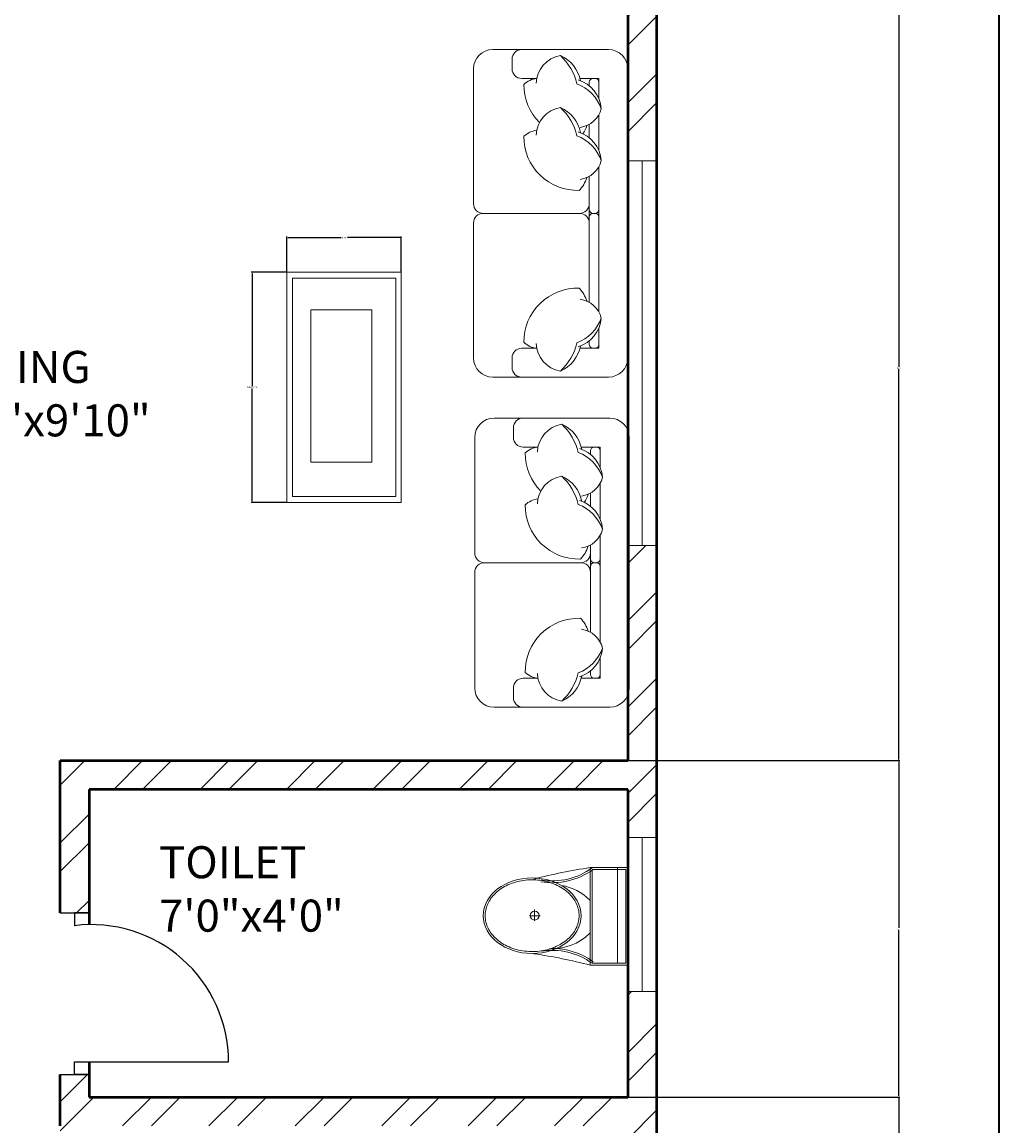
# Model space of a CAD drawing. Units: inches. Extents: x 2129 to 2642, y 1542 to 2414.
# Tile 8 of 9: x 2490 to 2642, y 2007 to 2179. Entities that reach past the tile are written whole.
import ezdxf

# ---------------------------------------------------------------- set-up
doc = ezdxf.new("R2010")
doc.units = ezdxf.units.IN
for name, color, linetype, lineweight in [('A-ANNO-DIMS', 2, 'Continuous', 18), ('A-ANNO-TTLB', 7, 'Continuous', 35), ('A-AREA-IDEN', 7, 'Continuous', 18), ('A-DOOR', 3, 'Continuous', 25), ('A-FLOR-FIXT', 9, 'Continuous', 18), ('A-FURN', 8, 'Continuous', 18), ('A-GLAZ', 4, 'Continuous', 18), ('A-WALL', 7, 'Continuous', 50), ('A-WALL-PATT', 252, 'Continuous', 13)]:
    doc.layers.add(name, color=color, linetype=linetype, lineweight=lineweight)
doc.styles.get("Standard").update_dxf_attribs({"font": 'arial.ttf'})
doc.dimstyles.get("Standard").update_dxf_attribs({"dimtxt": 0.18, "dimasz": 0.18, "dimexe": 0.18, "dimexo": 0.0625, "dimgap": 0.09, "dimtad": 0, "dimtih": 1, "dimtoh": 1, "dimdec": 4, "dimzin": 0, "dimdsep": 46, "dimtxsty": 'Standard', "dimcen": 0.09, "dimadec": 0, "dimazin": 0, "dimtfac": 1, "dimtdec": 4, "dimtofl": 0, "dimtmove": 0, "dimatfit": 3, "dimfxl": 1, "dimtolj": 1, "dimtzin": 0, "dimarcsym": 0})

# ---------------------------------------------------------------- blocks, each defined once
blk = doc.blocks.new('A$C31115884')
for p, q in [((283.1, 497.7), (223.4, 497.7)), ((257.5, 466.4), (257.5, 523.2)), ((0, 200), (0, 0)), ((520, 200), (0, 200)), ((10, 190), (10, 10)), ((510, 190), (10, 190)), ((510, 10), (510, 190)), ((520, 0), (520, 200)), ((510, 54.5), (0, 54.5)), ((10, 10), (510, 10)), ((0, 0), (520, 0))]:
    blk.add_line(p, q)
blk.add_circle((255.6, 496.4), 23.6)
for centre, radius, start, end in [((2777.7, -204.6), 2807, 165.4549, 171.71327), ((3237, 905), 2807, 188.28673, 194.5451), ((-294.5, 403.3), 364.7, 324.20913, 9.34987), ((-294.5, 403.3), 374.7, 324.20913, 9.34987), ((139.5, 406.2), 293.5, 315.84364, 2.65635), ((805.8, 403.3), 364.7, 170.65013, 215.79087), ((383.6, 406.2), 293.5, 190.27735, 224.15636), ((805.8, 403.3), 374.7, 179.20365, 215.79087)]:
    blk.add_arc(centre, radius, start, end)
blk.add_ellipse((256.2, 509.9), major_axis=(0, -260.7), ratio=0.772727)
blk.add_open_spline([(256.2, 259.2), (263.1, 259.2), (270, 259.7), (287.8, 262.3), (298.7, 265.1), (319.9, 273.1), (330.2, 278.4), (350.1, 291.1), (359.7, 298.7), (377.7, 315.9), (386.2, 325.5), (401.7, 346.6), (408.8, 358.1), (421.3, 382.5), (426.8, 395.5), (435.9, 422.4), (439.5, 436.4), (444.8, 465.1), (446.5, 479.7), (447.9, 509.2), (447.6, 524), (445, 553.3), (442.7, 567.8), (436.3, 596), (432.1, 609.7), (421.9, 636), (416, 648.6), (402.5, 672.1), (395, 683), (378.6, 703), (369.8, 712.1), (351.1, 728), (341.3, 734.8), (320.9, 746.2), (310.4, 750.7), (288.9, 757.3), (278, 759.4), (256, 761), (245, 760.6), (223.1, 757.2), (212.3, 754.3), (191.1, 746.1), (180.8, 740.7), (160.9, 727.8), (151.4, 720.1), (133.5, 702.7), (125.1, 693), (109.6, 671.7), (102.6, 660.2), (90.2, 635.7), (84.9, 622.7), (76, 595.6), (72.4, 581.6), (67.2, 552.9), (65.6, 538.2), (64.4, 508.8), (64.8, 494), (67.5, 464.7), (69.9, 450.2), (76.6, 422), (80.8, 408.3), (91.1, 382.2), (97.2, 369.7), (110.8, 346.3), (118.4, 335.4), (134.8, 315.6), (143.7, 306.7), (162.4, 290.9), (172.3, 284.2), (192.8, 273), (203.3, 268.6), (224.8, 262.2), (235.8, 260.2), (249.9, 259.3), (253, 259.2), (256.2, 259.2)], degree=3, knots=[0, 0, 0, 0, 0.110105, 0.110105, 0.285049, 0.285049, 0.459994, 0.459994, 0.634938, 0.634938, 0.809882, 0.809882, 0.984827, 0.984827, 1.159771, 1.159771, 1.334715, 1.334715, 1.50966, 1.50966, 1.684604, 1.684604, 1.859549, 1.859549, 2.034493, 2.034493, 2.209437, 2.209437, 2.384382, 2.384382, 2.559326, 2.559326, 2.73427, 2.73427, 2.909215, 2.909215, 3.084159, 3.084159, 3.259103, 3.259103, 3.434048, 3.434048, 3.608992, 3.608992, 3.783936, 3.783936, 3.958881, 3.958881, 4.133825, 4.133825, 4.30877, 4.30877, 4.483714, 4.483714, 4.658658, 4.658658, 4.833603, 4.833603, 5.008547, 5.008547, 5.183491, 5.183491, 5.358436, 5.358436, 5.53338, 5.53338, 5.708324, 5.708324, 5.883269, 5.883269, 6.058213, 6.058213, 6.233158, 6.233158, 6.283185, 6.283185, 6.283185, 6.283185])
blk = doc.blocks.new('TABLE-COFFEE')
for points in [[(0, 35.92), (17.84, 35.92), (17.84, 0), (0, 0)], [(0.86, 34.99), (17.01, 34.99), (17.01, 0.93), (0.86, 0.93)], [(3.74, 30.05), (13.25, 30.05), (13.25, 6.3), (3.74, 6.3)]]:
    blk.add_lwpolyline(points, close=True)
blk = doc.blocks.new('WIN-60-B')
for p, q in [((4.5, 60), (0, 60)), ((0, 60), (2.25, 60)), ((2.25, 60), (2.25, 0)), ((2.25, 0), (0, 0)), ((0, 0), (4.5, 0))]:
    blk.add_line(p, q)
blk = doc.blocks.new('*D32')
at = {"layer": 'A-ANNO-DIMS', "color": 0, "lineweight": -2, "transparency": 16777216}
for p, q in [((2531.18, 2140.41), (2525.67, 2140.41)), ((2525.85, 2140.23), (2525.85, 2122.64)), ((2525.85, 2104.67), (2525.85, 2122.27)), ((2531.18, 2104.49), (2525.67, 2104.49))]:
    blk.add_line(p, q, dxfattribs=at)
at = {"layer": 'A-ANNO-DIMS', "color": 0, "transparency": 16777216}
for points in [[(2525.82, 2140.23), (2525.88, 2140.23), (2525.85, 2140.41)], [(2525.82, 2104.67), (2525.88, 2104.67), (2525.85, 2104.49)]]:
    blk.add_solid(points, dxfattribs=at)
at = {"layer": 'Defpoints', "color": 0, "transparency": 16777216}
for p in [(2525.85, 2140.41), (2531.24, 2140.41), (2531.24, 2104.49)]:
    blk.add_point(p, dxfattribs=at)
at = {"layer": 'A-ANNO-DIMS', "color": 0, "transparency": 16777216, "insert": (2525.85, 2122.45), "char_height": 0.18, "attachment_point": 5}
blk.add_mtext('\\A1;TABLE 36 TYP.', dxfattribs=at)
blk = doc.blocks.new('*D33')
at = {"layer": 'A-ANNO-DIMS', "color": 0, "lineweight": -2, "transparency": 16777216}
for p, q in [((2531.24, 2140.48), (2531.24, 2145.98)), ((2531.42, 2145.8), (2539.64, 2145.8)), ((2548.91, 2145.8), (2540.68, 2145.8)), ((2549.09, 2140.48), (2549.09, 2145.98))]:
    blk.add_line(p, q, dxfattribs=at)
at = {"layer": 'A-ANNO-DIMS', "color": 0, "transparency": 16777216}
for points in [[(2531.42, 2145.83), (2531.42, 2145.77), (2531.24, 2145.8)], [(2548.91, 2145.83), (2548.91, 2145.77), (2549.09, 2145.8)]]:
    blk.add_solid(points, dxfattribs=at)
at = {"layer": 'Defpoints', "color": 0, "transparency": 16777216}
for p in [(2549.09, 2145.8), (2531.24, 2140.41), (2549.09, 2140.41)]:
    blk.add_point(p, dxfattribs=at)
at = {"layer": 'A-ANNO-DIMS', "color": 0, "transparency": 16777216, "insert": (2540.16, 2145.8), "char_height": 0.18, "attachment_point": 5}
blk.add_mtext('\\A1;18 TYP.', dxfattribs=at)
blk = doc.blocks.new('*D42')
at = {"layer": 'A-ANNO-DIMS', "color": 0, "lineweight": -2, "transparency": 16777216}
for p, q in [((2584.47, 2011.72), (2626.83, 2011.72)), ((2626.65, 2011.54), (2626.65, 1976.65)), ((2626.65, 1941.4), (2626.65, 1976.29)), ((2584.47, 1941.22), (2626.83, 1941.22))]:
    blk.add_line(p, q, dxfattribs=at)
at = {"layer": 'A-ANNO-DIMS', "color": 0, "transparency": 16777216}
for points in [[(2626.62, 2011.54), (2626.68, 2011.54), (2626.65, 2011.72)], [(2626.62, 1941.4), (2626.68, 1941.4), (2626.65, 1941.22)]]:
    blk.add_solid(points, dxfattribs=at)
at = {"layer": 'Defpoints', "color": 0, "transparency": 16777216}
for p in [(2584.4, 2011.72), (2626.65, 2011.72), (2584.4, 1941.22)]:
    blk.add_point(p, dxfattribs=at)
at = {"layer": 'A-ANNO-DIMS', "color": 0, "transparency": 16777216, "insert": (2626.65, 1976.47), "char_height": 0.18, "attachment_point": 5}
blk.add_mtext('\\A1;70.5', dxfattribs=at)
blk = doc.blocks.new('*D43')
at = {"layer": 'A-ANNO-DIMS', "color": 0, "lineweight": -2, "transparency": 16777216}
for p, q in [((2584.47, 2064.22), (2626.83, 2064.22)), ((2626.65, 2064.04), (2626.65, 2038.15)), ((2626.65, 2011.9), (2626.65, 2037.79)), ((2584.47, 2011.72), (2626.83, 2011.72))]:
    blk.add_line(p, q, dxfattribs=at)
at = {"layer": 'A-ANNO-DIMS', "color": 0, "transparency": 16777216}
for points in [[(2626.62, 2064.04), (2626.68, 2064.04), (2626.65, 2064.22)], [(2626.62, 2011.9), (2626.68, 2011.9), (2626.65, 2011.72)]]:
    blk.add_solid(points, dxfattribs=at)
at = {"layer": 'Defpoints', "color": 0, "transparency": 16777216}
for p in [(2584.4, 2064.22), (2626.65, 2064.22), (2584.4, 2011.72)]:
    blk.add_point(p, dxfattribs=at)
at = {"layer": 'A-ANNO-DIMS', "color": 0, "transparency": 16777216, "insert": (2626.65, 2037.97), "char_height": 0.18, "attachment_point": 5}
blk.add_mtext('\\A1;52.5', dxfattribs=at)
blk = doc.blocks.new('*D44')
at = {"layer": 'A-ANNO-DIMS', "color": 0, "lineweight": -2, "transparency": 16777216}
for p, q in [((2584.47, 2186.72), (2626.83, 2186.72)), ((2626.65, 2186.54), (2626.65, 2125.65)), ((2626.65, 2064.4), (2626.65, 2125.29)), ((2584.47, 2064.22), (2626.83, 2064.22))]:
    blk.add_line(p, q, dxfattribs=at)
at = {"layer": 'A-ANNO-DIMS', "color": 0, "transparency": 16777216}
for points in [[(2626.62, 2186.54), (2626.68, 2186.54), (2626.65, 2186.72)], [(2626.62, 2064.4), (2626.68, 2064.4), (2626.65, 2064.22)]]:
    blk.add_solid(points, dxfattribs=at)
at = {"layer": 'Defpoints', "color": 0, "transparency": 16777216}
for p in [(2584.4, 2186.72), (2626.65, 2186.72), (2584.4, 2064.22)]:
    blk.add_point(p, dxfattribs=at)
at = {"layer": 'A-ANNO-DIMS', "color": 0, "transparency": 16777216, "insert": (2626.65, 2125.47), "char_height": 0.18, "attachment_point": 5}
blk.add_mtext('\\A1;122.5', dxfattribs=at)

msp = doc.modelspace()

# ---------------------------------------------------------------- hatches: boundary and pattern name
at = {"layer": 'A-WALL-PATT'}
h = msp.add_hatch(dxfattribs=at)
h.set_pattern_fill('ANSI32', color=256)
h.paths.add_polyline_path([(2306.2606, 2305.9717), (2306.2606, 2308.2217), (2276.3515, 2308.2217), (2276.3515, 2303.7217), (2306.2606, 2303.7217)])
h.paths.add_polyline_path([(2216.3515, 2305.9717), (2216.3515, 2308.2217), (2186.9043, 2308.2217), (2186.9043, 2278.1696), (2191.4043, 2278.1696), (2191.4043, 2303.7217), (2216.3515, 2303.7217)])
h.paths.add_polyline_path([(2339.9043, 2335.7217), (2362.1938, 2335.7217), (2362.1938, 2340.2217), (2335.4043, 2340.2217), (2335.4043, 2308.2217), (2329.3487, 2308.2217), (2329.3487, 2305.9717), (2329.3487, 2303.7217), (2335.4043, 2303.7217), (2335.4043, 2186.7217), (2329.4345, 2186.7217), (2329.4345, 2182.2217), (2335.4043, 2182.2217), (2335.4043, 2174.7178), (2339.9043, 2174.7178), (2339.9043, 2182.2217), (2339.9043, 2303.7217)])
h.paths.add_polyline_path([(2440.4043, 2340.2217), (2411.654, 2340.2217), (2411.654, 2335.7217), (2435.9043, 2335.7217), (2435.9043, 2303.7217), (2435.9043, 2182.2217), (2435.9043, 2174.1935), (2438.1543, 2174.1935), (2440.4043, 2174.1935), (2440.4043, 2182.2217), (2444.653, 2182.2217), (2444.653, 2184.4717), (2444.653, 2186.7217), (2440.4043, 2186.7217), (2440.4043, 2303.7217), (2445.8547, 2303.7217), (2445.8547, 2308.2217), (2440.4043, 2308.2217)])
h.paths.add_polyline_path([(2498.2381, 2308.2217), (2470.3901, 2308.2217), (2470.3901, 2303.7217), (2498.2381, 2303.7217), (2498.2381, 2305.9717)])
h.paths.add_polyline_path([(2588.9043, 2308.2217), (2586.9043, 2308.2217), (2558.2381, 2308.2217), (2558.2381, 2303.7217), (2584.4043, 2303.7217), (2584.4043, 2279.1087), (2588.9043, 2279.1087)])
h.paths.add_polyline_path([(2588.9043, 2219.1087), (2584.4043, 2219.1087), (2584.4043, 2186.7217), (2478.0667, 2186.7217), (2478.0667, 2182.2217), (2584.4043, 2182.2217), (2584.4043, 2157.7883), (2588.9043, 2157.7883)])
h.paths.add_polyline_path([(2588.9043, 2097.7883), (2584.6063, 2097.7883), (2584.6063, 2075.5462, -0.09241561), (2584.4043, 2074.4627), (2584.4043, 2064.2217), (2495.9043, 2064.2217), (2495.9043, 2040.4611), (2500.4043, 2040.4611), (2500.4043, 2059.7217), (2584.4043, 2059.7217), (2584.4043, 2052.2164), (2588.9043, 2052.2164)])
h.paths.add_polyline_path([(2588.9043, 2028.2164), (2584.4043, 2028.2164), (2584.4043, 2011.7217), (2500.4043, 2011.7217), (2500.4043, 2015.243), (2498.1543, 2015.243), (2495.9043, 2015.243), (2495.9043, 2007.2217), (2495.9043, 2003.7597), (2500.4043, 2003.7597), (2500.4043, 2007.2217), (2584.4043, 2007.2217), (2584.4043, 1992.1997), (2588.9043, 1992.1997)])
h.paths.add_polyline_path([(2588.9043, 1956.1997), (2584.4043, 1956.1997), (2584.4043, 1941.2217), (2500.4043, 1941.2217), (2500.4043, 1985.1493), (2498.1543, 1985.1493), (2495.9043, 1985.1493), (2495.9043, 1941.2217), (2435.9043, 1941.2217), (2435.9043, 1930.3963), (2440.4043, 1930.3963), (2440.4043, 1936.7217), (2584.4043, 1936.7217), (2584.4043, 1909.8406), (2588.9043, 1909.8406)])
h.paths.add_polyline_path([(2588.9043, 1849.8406), (2584.4043, 1849.8406), (2584.4043, 1801.3526), (2588.9043, 1801.3526)])
h.paths.add_polyline_path([(2584.4043, 1828.7217), (2495.9043, 1828.7217), (2440.4043, 1828.7217), (2440.4043, 1905.2159), (2438.1543, 1905.2159), (2435.9043, 1905.2159), (2435.9043, 1828.7217), (2428.9101, 1828.7217), (2428.9101, 1824.2217), (2584.4043, 1824.2217)])
h.paths.add_polyline_path([(2588.9043, 1741.3526), (2584.4043, 1741.3526), (2584.4043, 1704.2217), (2468.3173, 1704.2217), (2468.3173, 1701.9717), (2468.3173, 1699.7217), (2588.9043, 1699.7217)])
h.paths.add_polyline_path([(2442.4043, 1761.7217), (2435.0216, 1761.7217), (2435.0216, 1757.2217), (2437.9043, 1757.2217), (2437.9043, 1665.7217), (2442.4043, 1665.7217), (2442.4043, 1667.7217), (2442.4043, 1699.7217), (2446.6907, 1699.7217), (2446.6907, 1701.9717), (2446.6907, 1704.2217), (2442.4043, 1704.2217)])
h.paths.add_polyline_path([(2390.4043, 1757.2217), (2410.8996, 1757.2217), (2410.8996, 1761.7217), (2360.1741, 1761.7217), (2360.1741, 1759.4717), (2360.1741, 1757.2217), (2385.9043, 1757.2217), (2385.9043, 1674.8326), (2390.4043, 1674.8326)])
h.paths.add_polyline_path([(2337.9043, 1757.2217), (2340.3592, 1757.2217), (2340.3592, 1759.4717), (2340.3592, 1761.7217), (2333.4043, 1761.7217), (2333.4043, 1704.2217), (2327.381, 1704.2217), (2327.381, 1701.9717), (2327.381, 1699.7217), (2333.4043, 1699.7217), (2333.4043, 1665.7217), (2337.9043, 1665.7217)])
h.paths.add_polyline_path([(2191.4043, 1743.4804), (2186.9043, 1743.4804), (2186.9043, 1699.7217), (2188.9043, 1699.7217), (2191.4043, 1699.7217), (2306.5617, 1699.7217), (2306.5617, 1704.2217), (2191.4043, 1704.2217)])
h.paths.add_polyline_path([(2191.4043, 1859.8992), (2186.9043, 1859.8992), (2186.9043, 1803.4804), (2189.1543, 1803.4804), (2191.4043, 1803.4804)])
h.paths.add_polyline_path([(2352.5445, 1828.7217), (2191.4043, 1828.7217), (2191.4043, 1824.2217), (2333.4043, 1824.2217), (2352.5445, 1824.2217), (2352.5445, 1826.4717)])
h.paths.add_polyline_path([(2390.4043, 2085.328), (2385.9043, 2085.328), (2385.9043, 1828.7217), (2381.9668, 1828.7217), (2381.9668, 1826.4717), (2381.9668, 1824.2217), (2385.9043, 1824.2217), (2385.9043, 1761.7217), (2390.4043, 1761.7217), (2390.4043, 1824.2217), (2394.1868, 1824.2217), (2394.1868, 1827.6339), (2394.1868, 1828.7217), (2390.4043, 1828.7217)])
h.paths.add_polyline_path([(2339.9043, 1941.2217), (2335.4043, 1941.2217), (2279.9043, 1941.2217), (2279.9043, 1981.3432), (2277.6543, 1981.3432), (2275.4043, 1981.3432), (2275.4043, 1941.2217), (2191.4043, 1941.2217), (2191.4043, 1958.1079), (2186.9043, 1958.1079), (2186.9043, 1919.8992), (2189.1543, 1919.8992), (2191.4043, 1919.8992), (2191.4043, 1936.7217), (2279.9043, 1936.7217), (2335.4043, 1936.7217), (2335.4043, 1931.1382), (2339.9043, 1931.1382)])
h.paths.add_polyline_path([(2339.9043, 1902.7544), (2337.6543, 1902.7544), (2335.4043, 1902.7544), (2335.4043, 1828.7217), (2339.9043, 1828.7217)])
h.paths.add_polyline_path([(2279.9043, 2015.263), (2277.6543, 2015.263), (2275.4043, 2015.263), (2275.4043, 2011.7217), (2191.4043, 2011.7217), (2191.4043, 2026.6781), (2186.9043, 2026.6781), (2186.9043, 1994.1079), (2189.1543, 1994.1079), (2191.4043, 1994.1079), (2191.4043, 2007.2217), (2275.4043, 2007.2217), (2275.4043, 2003.2288), (2279.9043, 2003.2288), (2279.9043, 2007.2217)])
h.paths.add_polyline_path([(2296.0216, 2186.7217), (2191.4043, 2186.7217), (2191.4043, 2218.1696), (2186.9043, 2218.1696), (2186.9043, 2158.4509), (2191.4043, 2158.4509), (2191.4043, 2182.2217), (2296.0216, 2182.2217), (2296.0216, 2184.4717)])
h.paths.add_polyline_path([(2191.4043, 2098.4509), (2189.1543, 2098.4509), (2186.9043, 2098.4509), (2186.9043, 2050.6781), (2189.0487, 2050.6781), (2191.4043, 2050.6781), (2191.4043, 2059.7217), (2275.4043, 2059.7217), (2275.4043, 2038.4133), (2279.9043, 2038.4133), (2279.9043, 2064.2217), (2191.4043, 2064.2217)])
h.paths.add_polyline_path([(2268.3923, 1605.9386), (2516.3159, 1605.9386), (2516.3159, 1643.0314), (2268.3923, 1643.0314)], flags=9)
h.paths.add_polyline_path([(2399.6079, 1710.4489), (2428.8405, 1710.4489), (2428.8405, 1729.1062), (2399.6079, 1729.1062)], flags=9)
h.paths.add_polyline_path([(2342.1483, 1708.9956), (2371.3809, 1708.9956), (2371.3809, 1727.653), (2342.1483, 1727.653)], flags=9)
h.paths.add_polyline_path([(2200.7404, 1677.2519), (2282.3059, 1677.2519), (2282.3059, 1687.5555), (2200.7404, 1687.5555)], flags=9)
h.paths.add_polyline_path([(2209.8153, 1704.7448), (2250.627, 1704.7448), (2250.627, 1723.4021), (2209.8153, 1723.4021)], flags=25)
h.paths.add_polyline_path([(2213.9996, 1911.284), (2252.84, 1911.284), (2252.84, 1929.9413), (2213.9996, 1929.9413)], flags=9)
h.paths.add_polyline_path([(2210.8865, 1962.0987), (2244.0447, 1962.0987), (2244.0447, 1980.7561), (2210.8865, 1980.7561)], flags=25)
h.paths.add_polyline_path([(2219.0745, 2037.6131), (2248.2321, 2037.6131), (2248.2321, 2056.2705), (2219.0745, 2056.2705)], flags=9)
h.paths.add_polyline_path([(2379.9702, 2099.0686), (2409.3767, 2099.0686), (2409.3767, 2117.7259), (2379.9702, 2117.7259)], flags=9)
h.paths.add_polyline_path([(2375.9312, 2160.3752), (2405.3173, 2160.3752), (2405.3173, 2179.0325), (2375.9312, 2179.0325)], flags=9)
h.paths.add_polyline_path([(2269.5058, 2112.1824), (2310.3175, 2112.1824), (2310.3175, 2130.8397), (2269.5058, 2130.8397)], flags=9)
h.paths.add_polyline_path([(2209.6567, 2193.667), (2248.4971, 2193.667), (2248.4971, 2212.3243), (2209.6567, 2212.3243)], flags=25)
h.paths.add_polyline_path([(2491.6289, 1675.447), (2573.1944, 1675.447), (2573.1944, 1685.7506), (2491.6289, 1685.7506)], flags=9)
h.paths.add_polyline_path([(2492.0585, 1710.4489), (2530.8989, 1710.4489), (2530.8989, 1729.1062), (2492.0585, 1729.1062)], flags=25)
h.paths.add_polyline_path([(2495.6634, 1908.8646), (2534.5038, 1908.8646), (2534.5038, 1927.522), (2495.6634, 1927.522)], flags=9)
h.paths.add_polyline_path([(2516.7779, 1955.9942), (2549.9362, 1955.9942), (2549.9362, 1974.6516), (2516.7779, 1974.6516)], flags=25)
h.paths.add_polyline_path([(2509.7444, 2034.6896), (2538.902, 2034.6896), (2538.902, 2053.347), (2509.7444, 2053.347)], flags=9)
h.paths.add_polyline_path([(2467.8454, 2111.9593), (2508.6571, 2111.9593), (2508.6571, 2130.6167), (2467.8454, 2130.6167)], flags=9)
h.paths.add_polyline_path([(2528.5267, 2189.1742), (2567.3671, 2189.1742), (2567.3671, 2207.8316), (2528.5267, 2207.8316)], flags=25)
h.paths.add_polyline_path([(2483.7603, 2319.9841), (2557.5563, 2319.9841), (2557.5563, 2330.2877), (2483.7603, 2330.2877)], flags=9)
h.paths.add_polyline_path([(2204.078, 2317.0445), (2277.874, 2317.0445), (2277.874, 2327.3481), (2204.078, 2327.3481)], flags=9)

# ---------------------------------------------------------------- linework, layer by layer
at = {"layer": 'A-ANNO-TTLB'}
msp.add_lwpolyline([(2129.4387, 2413.7704), (2642.2731, 2413.7704), (2642.2731, 1542.3836), (2129.4387, 1542.3836)], close=True, dxfattribs=at)
at = {"layer": 'A-DOOR'}
for p, q in [((2495.9043, 2040.4611), (2500.4043, 2040.4611)), ((2500.4043, 2040.4611), (2498.1543, 2040.4611)), ((2498.1543, 2040.4611), (2498.1543, 2038.4611)), ((2498.1543, 2015.243), (2498.1543, 2017.243)), ((2498.1543, 2017.243), (2522.1543, 2017.243)), ((2495.9043, 2015.243), (2500.4043, 2015.243)), ((2500.4043, 2015.243), (2498.1543, 2015.243))]:
    msp.add_line(p, q, dxfattribs=at)
msp.add_arc((2500.775, 2017.243), 21.3793, 0, 97.041006, dxfattribs=at)
at = {"layer": 'A-FURN', "ltscale": 0.03}
for points in [[(2560.3497, 2148.0866, -0.41421356), (2561.8532, 2149.59, -0.41421356), (2560.3497, 2151.0935), (2560.3497, 2172.1412, -0.41421356), (2563.3566, 2175.1481), (2581.3975, 2175.1481, -0.41421356), (2584.4043, 2172.1412), (2584.4043, 2127.0388, -0.41421356), (2581.3975, 2124.032), (2563.3566, 2124.032, -0.41421356), (2560.3497, 2127.0388), (2560.3497, 2148.0866, -0.41421356), (2561.8532, 2149.59, -0.41421356), (2560.3497, 2151.0935)], [(2560.5517, 2093.5871, -0.41421356), (2562.0551, 2095.0905, -0.41421356), (2560.5517, 2096.594), (2560.5517, 2114.6349, -0.41421356), (2563.5585, 2117.6417), (2581.5995, 2117.6417, -0.41421356), (2584.6063, 2114.6349), (2584.6063, 2075.5462, -0.41421356), (2581.5995, 2072.5394), (2563.5585, 2072.5394, -0.41421356), (2560.5517, 2075.5462), (2560.5517, 2093.5871, -0.41421356), (2562.0551, 2095.0905, -0.41421356), (2560.5517, 2096.594)]]:
    msp.add_lwpolyline(points, format="xyb", dxfattribs=at)
at = {"layer": 'A-FURN'}
for points in [[(2570.1961, 2170.6378), (2567.8668, 2170.6378, -0.41421356), (2566.3634, 2172.1412), (2566.3634, 2173.6446, -0.41421356), (2567.8668, 2175.1481)], [(2570.1052, 2169.8833, -0.35677236), (2573.8947, 2174.1912, -0.24954205), (2577.0176, 2170.2879, 9.61688035)], [(2573.8947, 2174.1912, -0.14772988), (2576.4784, 2169.7972, -0.21334276), (2580.268, 2165.9201, -0.17866181)], [(2570.1968, 2170.6411, 0.16554063), (2568.2104, 2169.711, 0.20023115), (2570.6297, 2163.743, 0.12152332)], [(2576.6844, 2170.4042, -0.30666349), (2580.268, 2165.9201, -0.30632997), (2576.9952, 2162.9907, 0.87284716)], [(2579.8941, 2167.4751), (2579.8941, 2170.6378), (2576.9395, 2170.6378, -0.41421356)], [(2578.3907, 2169.4905), (2578.3907, 2170.0365, -0.41421356), (2578.9921, 2170.6378), (2579.2927, 2170.6378, -0.41421356), (2579.8941, 2170.0365)], [(2579.8941, 2170.0365), (2579.8941, 2167.4751, -0.41421356)], [(2570.1052, 2161.7845, -0.35677236), (2573.8947, 2166.0924, -0.24954205), (2577.0176, 2162.1891, 9.61688035)], [(2573.8947, 2166.0924, -0.14772988), (2576.4784, 2161.6984, -0.21334276), (2580.268, 2157.8213, -0.17866181)], [(2579.8941, 2164.9739), (2579.8941, 2159.3762, -0.41421356)], [(2577.4223, 2162.0114, 0.07186538), (2578.01, 2163.2719, -7.11546429)], [(2578.3907, 2161.3917), (2578.3907, 2163.4601, -0.41421356)], [(2570.1968, 2162.5423, 0.16554063), (2568.2104, 2161.6122, 0.42598917), (2576.8229, 2153.1687, 0.12152332), (2578.01, 2155.1731, -7.11546429)], [(2576.6844, 2162.3054, -0.30666349), (2580.268, 2157.8213, -0.30632997), (2576.9952, 2154.8919, 0.87284716)], [(2579.8941, 2156.8751), (2579.8941, 2150.1914, -0.41421356), (2579.2927, 2149.59), (2578.9921, 2149.59, -0.41421356), (2578.3907, 2150.1914), (2578.3907, 2155.3612, -0.41421356)], [(2578.3907, 2151.0935, -0.41421356), (2576.8873, 2149.59), (2561.8532, 2149.59, -0.41421356)], [(2578.3907, 2151.0935, -0.41421356), (2576.8873, 2149.59)], [(2578.3907, 2148.0866, 0.41421356), (2576.8873, 2149.59), (2561.8532, 2149.59, 0.41421356)], [(2578.3907, 2148.0866, 0.41421356), (2576.8873, 2149.59)], [(2579.8941, 2134.2062), (2579.8941, 2148.9887, 0.41421356), (2579.2927, 2149.59), (2578.9921, 2149.59, 0.41421356), (2578.3907, 2148.9887), (2578.3907, 2135.72, 0.41421356)], [(2570.1968, 2128.539, -0.16554063), (2568.2104, 2129.469, -0.42598917), (2576.8229, 2137.9125, -0.12152332), (2578.01, 2135.9082, 7.11546429)], [(2576.6844, 2128.7758, 0.30666349), (2580.268, 2133.26, 0.30632997), (2576.9952, 2136.1893, -0.87284716)], [(2573.8947, 2124.9888, 0.14772988), (2576.4784, 2129.3829, 0.21334276), (2580.268, 2133.26, 0.17866181)], [(2579.8941, 2129.1436), (2579.8941, 2131.705, 0.41421356)], [(2567.8668, 2124.032, -0.41421356), (2566.3634, 2125.5354), (2566.3634, 2127.0388, -0.41421356), (2567.8668, 2128.5423), (2570.1961, 2128.5423)], [(2570.1052, 2129.2967, 0.35677236), (2573.8947, 2124.9888, 0.24954205), (2577.0176, 2128.8922, -9.61688035)], [(2578.3907, 2129.6895), (2578.3907, 2129.1436, 0.41421356), (2578.9921, 2128.5423), (2579.2927, 2128.5423, 0.41421356), (2579.8941, 2129.1436)], [(2570.3981, 2113.1315), (2568.0688, 2113.1315, -0.41421356), (2566.5654, 2114.6349), (2566.5654, 2116.1383, -0.41421356), (2568.0688, 2117.6417)], [(2570.3071, 2112.377, -0.35677236), (2574.0967, 2116.6849, -0.24954205), (2577.2195, 2112.7816, 9.61688035)], [(2574.0967, 2116.6849, -0.14772988), (2576.6804, 2112.2909, -0.21334276), (2580.4699, 2108.4138, -0.17866181)], [(2570.3988, 2113.1348, 0.16554063), (2568.4124, 2112.2047, 0.20023115), (2570.8316, 2106.2367, 0.12152332)], [(2580.0961, 2109.9687), (2580.0961, 2113.1315), (2577.1415, 2113.1315, -0.41421356)], [(2578.5927, 2111.9842), (2578.5927, 2112.5301, -0.41421356), (2579.194, 2113.1315), (2579.4947, 2113.1315, -0.41421356), (2580.0961, 2112.5301)], [(2576.8863, 2112.8979, -0.30666349), (2580.4699, 2108.4138, -0.30632997), (2577.1972, 2105.4844, 0.87284716)], [(2580.0961, 2112.5301), (2580.0961, 2109.9687, -0.41421356)], [(2570.3071, 2104.2782, -0.35677236), (2574.0967, 2108.5861, -0.24954205), (2577.2195, 2104.6827, 9.61688035)], [(2574.0967, 2108.5861, -0.14772988), (2576.6804, 2104.192, -0.21334276), (2580.4699, 2100.3149, -0.17866181)], [(2580.0961, 2107.4676), (2580.0961, 2101.8699, -0.41421356)], [(2570.3988, 2105.0359, 0.16554063), (2568.4124, 2104.1059, 0.42598917), (2577.0249, 2095.6624, 0.12152332), (2578.212, 2097.6667, -7.11546429)], [(2576.8863, 2104.7991, -0.30666349), (2580.4699, 2100.3149, -0.30632997), (2577.1972, 2097.3856, 0.87284716)], [(2577.6243, 2104.5051, 0.07186538), (2578.212, 2105.7656, -7.11546429)], [(2578.5927, 2103.8854), (2578.5927, 2105.9538, -0.41421356)], [(2580.0961, 2099.3688), (2580.0961, 2095.6919, -0.41421356), (2579.4947, 2095.0905), (2579.194, 2095.0905, -0.41421356), (2578.5927, 2095.6919), (2578.5927, 2097.8549, -0.41421356)], [(2578.5927, 2096.594, -0.41421356), (2577.0893, 2095.0905), (2562.0551, 2095.0905, -0.41421356)], [(2578.5927, 2096.594, -0.41421356), (2577.0893, 2095.0905)], [(2578.5927, 2093.5871, 0.41421356), (2577.0893, 2095.0905), (2562.0551, 2095.0905, 0.41421356)], [(2578.5927, 2093.5871, 0.41421356), (2577.0893, 2095.0905)], [(2580.0961, 2082.7135), (2580.0961, 2094.4892, 0.41421356), (2579.4947, 2095.0905), (2579.194, 2095.0905, 0.41421356), (2578.5927, 2094.4892), (2578.5927, 2084.2273, 0.41421356)], [(2570.3988, 2077.0463, -0.16554063), (2568.4124, 2077.9764, -0.42598917), (2577.0249, 2086.4198, -0.12152332), (2578.212, 2084.4155, 7.11546429)], [(2576.8863, 2077.2832, 0.30666349), (2580.4699, 2081.7673, 0.30632997), (2577.1972, 2084.6967, -0.87284716)], [(2574.0967, 2073.4962, 0.14772988), (2576.6804, 2077.8902, 0.21334276), (2580.4699, 2081.7673, 0.17866181)], [(2580.0961, 2077.651), (2580.0961, 2080.2124, 0.41421356)], [(2568.0688, 2072.5394, -0.41421356), (2566.5654, 2074.0428), (2566.5654, 2075.5462, -0.41421356), (2568.0688, 2077.0496), (2570.3981, 2077.0496)], [(2570.3071, 2077.8041, 0.35677236), (2574.0967, 2073.4962, 0.24954205), (2577.2195, 2077.3995, -9.61688035)], [(2578.5927, 2078.1969), (2578.5927, 2077.651, 0.41421356), (2579.194, 2077.0496), (2579.4947, 2077.0496, 0.41421356), (2580.0961, 2077.651)]]:
    msp.add_lwpolyline(points, format="xyb", dxfattribs=at)
for points in [[(2579.8941, 2159.3762), (2579.8941, 2164.9739)], [(2579.8941, 2134.2062), (2579.8941, 2156.8751)], [(2576.9395, 2128.5423), (2579.8941, 2128.5423), (2579.8941, 2131.705)], [(2580.0961, 2101.8699), (2580.0961, 2107.4676)], [(2580.0961, 2082.7135), (2580.0961, 2099.3688)], [(2577.1415, 2077.0496), (2580.0961, 2077.0496), (2580.0961, 2080.2124)]]:
    msp.add_lwpolyline(points, dxfattribs=at)
for points in [[(2579.8941, 2148.9887), (2579.8941, 2150.1914, -0.41421356), (2579.2927, 2149.59), (2578.9921, 2149.59, -0.41421356), (2578.3907, 2150.1914), (2578.3907, 2148.9887, -0.41421356), (2578.9921, 2149.59), (2579.2927, 2149.59, -0.41421356)], [(2580.0961, 2094.4892), (2580.0961, 2095.6919, -0.41421356), (2579.4947, 2095.0905), (2579.194, 2095.0905, -0.41421356), (2578.5927, 2095.6919), (2578.5927, 2094.4892, -0.41421356), (2579.194, 2095.0905), (2579.4947, 2095.0905, -0.41421356)]]:
    msp.add_lwpolyline(points, format="xyb", close=True, dxfattribs=at)
msp.add_lwpolyline([(2531.2429, 2140.4141), (2549.0856, 2140.4141), (2549.0856, 2104.4925), (2531.2429, 2104.4925)], close=True, dxfattribs=at)
at = {"layer": 'A-GLAZ'}
for p, q in [((2584.4043, 2052.2164), (2588.9043, 2052.2164)), ((2588.9043, 2052.2164), (2586.6543, 2052.2164)), ((2586.6543, 2052.2164), (2586.6543, 2028.2164)), ((2586.6543, 2028.2164), (2584.4043, 2028.2164)), ((2584.4043, 2028.2164), (2588.9043, 2028.2164))]:
    msp.add_line(p, q, dxfattribs=at)
at = {"layer": 'A-WALL'}
for p, q in [((2588.9043, 2308.2217), (2588.9043, 1699.7217)), ((2584.4043, 2182.2217), (2584.4043, 2064.2217)), ((2495.9043, 2064.2217), (2584.4043, 2064.2217)), ((2495.9043, 2040.4611), (2495.9043, 2064.2217)), ((2584.4043, 2059.7217), (2500.4043, 2059.7217)), ((2584.4043, 2059.7217), (2500.4043, 2059.7217)), ((2500.4043, 2059.7217), (2500.4043, 2038.6191)), ((2584.4043, 2059.7217), (2584.4043, 2011.7217)), ((2500.4043, 2017.243), (2500.4043, 2011.7217)), ((2495.9043, 2007.2217), (2495.9043, 2015.243)), ((2500.4043, 2011.7217), (2584.4043, 2011.7217))]:
    msp.add_line(p, q, dxfattribs=at)

# ---------------------------------------------------------------- block references
at = {"layer": 'A-FLOR-FIXT', "xscale": -0.0292470664339069, "yscale": 0.0292470664339069, "zscale": 0.0292470664339069, "rotation": 90}
msp.add_blockref('A$C31115884', (2584.4043, 2047.5127), dxfattribs=at)
at = {"layer": 'A-FURN'}
msp.add_blockref('TABLE-COFFEE', (2531.2426, 2104.4928), dxfattribs=at)
at = {"layer": 'A-GLAZ', "rotation": 180}
msp.add_blockref('WIN-60-B', (2588.9047, 2157.7887), dxfattribs=at)

# ---------------------------------------------------------------- texts
at = {"layer": 'A-AREA-IDEN', "char_height": 5, "attachment_point": 1}
for s, width, insert in [('DRAWING\\P11\'10"x9\'10"', 102.911185, (2469.8559, 2128.1286)), ('TOILET\\P7\'0"x4\'0"', 89.415082, (2511.3252, 2050.8623))]:
    msp.add_mtext_dynamic_manual_height_columns(s, width=width, gutter_width=12.5, heights=[0], dxfattribs=dict(at, insert=insert))

# ---------------------------------------------------------------- dimensions: what is measured, and where the dimension line sits
at = {"layer": 'A-ANNO-DIMS'}
for base, p1, p2, picture, middle in [((2626.6543, 2186.7217), (2584.4043, 2064.2217), (2584.4043, 2186.7217), '*D44', (2626.6543, 2125.4717)), ((2626.6543, 2064.2217), (2584.4043, 2011.7217), (2584.4043, 2064.2217), '*D43', (2626.6543, 2037.9717)), ((2626.6543, 2011.7217), (2584.4043, 1941.2217), (2584.4043, 2011.7217), '*D42', (2626.6543, 1976.4717))]:
    dim = msp.add_linear_dim(base=base, p1=p1, p2=p2, angle=90, dimstyle='Standard', override={"dimdec": 1, "dimlfac": 1, "dimrnd": 0, "dimzin": 0, "dimdsep": 46, "dimlunit": 2}, dxfattribs=at)
    dim.commit()
    dim.dimension.update_dxf_attribs({"geometry": picture, "text_midpoint": middle})
dim = msp.add_linear_dim(base=(2549.0856, 2145.8024), p1=(2531.2429, 2140.4141), p2=(2549.0856, 2140.4141), text='<> TYP.', dimstyle='Standard', override={"dimdec": 0, "dimlfac": 1, "dimrnd": 0, "dimzin": 0, "dimdsep": 46, "dimlunit": 2}, dxfattribs=at)
dim.commit()
dim.dimension.update_dxf_attribs({"geometry": '*D33', "text_midpoint": (2540.1643, 2145.8024)})
dim = msp.add_linear_dim(base=(2525.8546, 2140.4141), p1=(2531.2429, 2104.4925), p2=(2531.2429, 2140.4141), angle=90, text='TABLE <> TYP.', dimstyle='Standard', override={"dimdec": 0, "dimlfac": 1, "dimrnd": 0, "dimzin": 0, "dimdsep": 46, "dimlunit": 2}, dxfattribs=at)
dim.commit()
dim.dimension.update_dxf_attribs({"geometry": '*D32', "text_midpoint": (2525.8546, 2122.4533)})

doc.saveas('drawing.dxf')
